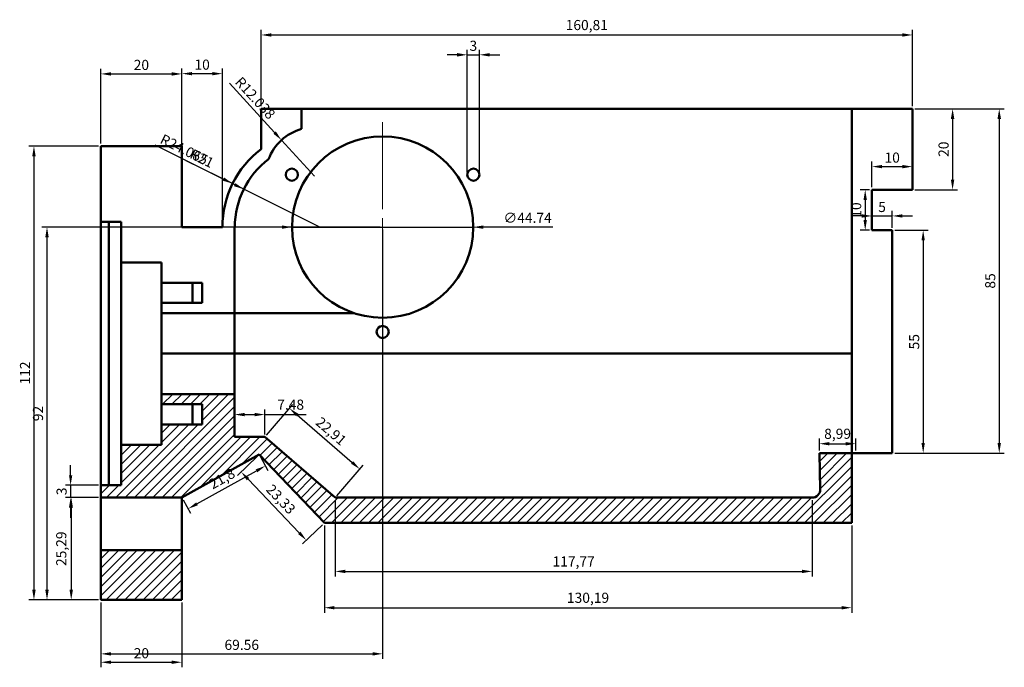
# Model space of a CAD drawing. Units: millimetres. Extents: x 1194 to 1920, y 1729 to 2086.
# Tile 1 of 5: x 1237 to 1480, y 1732 to 1891. Entities that reach past the tile are written whole.
import ezdxf

# ---------------------------------------------------------------- set-up
doc = ezdxf.new("R2010")
doc.units = ezdxf.units.MM
doc.linetypes.add('CENTER', pattern=[50.8, 31.75, -6.35, 6.35, -6.35])
for name, color, linetype, lineweight in [('M-CNTR', 1, 'CENTER', 18), ('M-DIMS', 2, 'Continuous', 25), ('M-HATC', 8, 'Continuous', 18), ('M-OUTL', 7, 'Continuous', 50)]:
    doc.layers.add(name, color=color, linetype=linetype, lineweight=lineweight)
doc.styles.get("Standard").update_dxf_attribs({"font": 'arial.ttf'})
doc.dimstyles.new('ISO-25', dxfattribs={"dimtxt": 2.5, "dimasz": 2.5, "dimexe": 1.25, "dimexo": 0.625, "dimtad": 1, "dimtxsty": 'Standard', "dimcen": 2.5, "dimadec": 0, "dimazin": 0, "dimtfac": 1, "dimtmove": 0, "dimatfit": 3, "dimfxl": 1, "dimarcsym": 0})

# ---------------------------------------------------------------- blocks, each defined once
blk = doc.blocks.new('*U10')
at = {"layer": 'M-CNTR', "color": 0, "transparency": 16777216}
for p, q in [((0, 4.47), (0, 25.87)), ((-25.87, 0), (-4.47, 0)), ((4.47, 0), (25.87, 0)), ((0, -25.87), (0, -4.47))]:
    blk.add_line(p, q, dxfattribs=at)
at = {"layer": 'M-CNTR', "color": 0, "linetype": 'Continuous', "transparency": 16777216}
for p, q in [((-2.24, 0), (2.24, 0)), ((0, -2.24), (0, 2.24))]:
    blk.add_line(p, q, dxfattribs=at)
blk = doc.blocks.new('*U11')
blk.add_circle((0, 0), 1.5)
blk = doc.blocks.new('*U12')
at = {"layer": 'M-OUTL', "color": 0, "linetype": 'ByBlock', "lineweight": -2, "transparency": 16777216}
for p, rotation in [((1304.02, 1853.17), 240), ((1348.83, 1853.17), 119.9999999999999)]:
    blk.add_blockref('*U11', p, dxfattribs=dict(at, rotation=rotation))
blk.add_blockref('*U11', (1326.43, 1814.36), dxfattribs=at)
blk = doc.blocks.new('*D81')
at = {"layer": 'Defpoints', "color": 0, "transparency": 16777216}
for p in [(1256.87, 1860.23), (1240.35, 1748.23), (1256.87, 1748.23)]:
    blk.add_point(p, dxfattribs=at)
at = {"layer": 'M-DIMS', "color": 0, "lineweight": -2, "transparency": 16777216}
for p, q in [((1256.25, 1860.23), (1239.1, 1860.23)), ((1240.35, 1857.73), (1240.35, 1750.73)), ((1256.25, 1748.23), (1239.1, 1748.23))]:
    blk.add_line(p, q, dxfattribs=at)
at = {"layer": 'M-DIMS', "color": 0, "transparency": 16777216}
for points in [[(1239.93, 1857.73), (1240.76, 1857.73), (1240.35, 1860.23)], [(1239.93, 1750.73), (1240.76, 1750.73), (1240.35, 1748.23)]]:
    blk.add_solid(points, dxfattribs=at)
at = {"layer": 'M-DIMS', "color": 0, "transparency": 16777216, "insert": (1238.47, 1804.23), "char_height": 2.5, "attachment_point": 5, "rotation": 90}
blk.add_mtext('112', dxfattribs=at)
blk = doc.blocks.new('*D82')
at = {"layer": 'Defpoints', "color": 0, "transparency": 16777216}
for p in [(1276.87, 1878.03), (1256.87, 1860.23), (1276.87, 1860.23)]:
    blk.add_point(p, dxfattribs=at)
at = {"layer": 'M-DIMS', "color": 0, "lineweight": -2, "transparency": 16777216}
for p, q in [((1256.87, 1860.86), (1256.87, 1879.28)), ((1276.87, 1860.86), (1276.87, 1879.28)), ((1259.37, 1878.03), (1274.37, 1878.03))]:
    blk.add_line(p, q, dxfattribs=at)
at = {"layer": 'M-DIMS', "color": 0, "transparency": 16777216}
for points in [[(1259.37, 1878.45), (1259.37, 1877.61), (1256.87, 1878.03)], [(1274.37, 1878.45), (1274.37, 1877.61), (1276.87, 1878.03)]]:
    blk.add_solid(points, dxfattribs=at)
at = {"layer": 'M-DIMS', "color": 0, "transparency": 16777216, "insert": (1266.87, 1879.93), "char_height": 2.5, "attachment_point": 5}
blk.add_mtext('20', dxfattribs=at)
blk = doc.blocks.new('*D83')
at = {"layer": 'Defpoints', "color": 0, "transparency": 16777216}
for p in [(1457.23, 1887.64), (1296.43, 1869.45), (1457.23, 1869.45)]:
    blk.add_point(p, dxfattribs=at)
at = {"layer": 'M-DIMS', "color": 0, "lineweight": -2, "transparency": 16777216}
for p, q in [((1296.43, 1870.07), (1296.43, 1888.89)), ((1457.23, 1870.07), (1457.23, 1888.89)), ((1298.93, 1887.64), (1454.73, 1887.64))]:
    blk.add_line(p, q, dxfattribs=at)
at = {"layer": 'M-DIMS', "color": 0, "transparency": 16777216}
for points in [[(1298.93, 1888.06), (1298.93, 1887.23), (1296.43, 1887.64)], [(1454.73, 1888.06), (1454.73, 1887.23), (1457.23, 1887.64)]]:
    blk.add_solid(points, dxfattribs=at)
at = {"layer": 'M-DIMS', "color": 0, "transparency": 16777216, "insert": (1376.83, 1889.77), "char_height": 2.5, "attachment_point": 5}
blk.add_mtext('160,81', dxfattribs=at)
blk = doc.blocks.new('*D84')
at = {"layer": 'Defpoints', "color": 0, "transparency": 16777216}
for p in [(1286.87, 1878.1), (1276.87, 1840.23), (1286.87, 1840.23)]:
    blk.add_point(p, dxfattribs=at)
at = {"layer": 'M-DIMS', "color": 0, "lineweight": -2, "transparency": 16777216}
for p, q in [((1276.87, 1840.86), (1276.87, 1879.35)), ((1286.87, 1840.86), (1286.87, 1879.35)), ((1279.37, 1878.1), (1284.37, 1878.1))]:
    blk.add_line(p, q, dxfattribs=at)
at = {"layer": 'M-DIMS', "color": 0, "transparency": 16777216}
for points in [[(1279.37, 1878.51), (1279.37, 1877.68), (1276.87, 1878.1)], [(1284.37, 1878.51), (1284.37, 1877.68), (1286.87, 1878.1)]]:
    blk.add_solid(points, dxfattribs=at)
at = {"layer": 'M-DIMS', "color": 0, "transparency": 16777216, "insert": (1281.87, 1880), "char_height": 2.5, "attachment_point": 5}
blk.add_mtext('10', dxfattribs=at)
blk = doc.blocks.new('*D85')
at = {"layer": 'Defpoints', "color": 0, "transparency": 16777216}
for p in [(1256.87, 1748.23), (1276.87, 1748.23), (1276.87, 1732.86)]:
    blk.add_point(p, dxfattribs=at)
at = {"layer": 'M-DIMS', "color": 0, "lineweight": -2, "transparency": 16777216}
for p, q in [((1256.87, 1747.61), (1256.87, 1731.61)), ((1276.87, 1747.61), (1276.87, 1731.61)), ((1259.37, 1732.86), (1274.37, 1732.86))]:
    blk.add_line(p, q, dxfattribs=at)
at = {"layer": 'M-DIMS', "color": 0, "transparency": 16777216}
for points in [[(1259.37, 1733.28), (1259.37, 1732.45), (1256.87, 1732.86)], [(1274.37, 1733.28), (1274.37, 1732.45), (1276.87, 1732.86)]]:
    blk.add_solid(points, dxfattribs=at)
at = {"layer": 'M-DIMS', "color": 0, "transparency": 16777216, "insert": (1266.87, 1734.77), "char_height": 2.5, "attachment_point": 5}
blk.add_mtext('20', dxfattribs=at)
blk = doc.blocks.new('*D86')
at = {"layer": 'Defpoints', "color": 0, "transparency": 16777216}
for p in [(1256.87, 1773.52), (1249.55, 1748.23), (1256.87, 1748.23)]:
    blk.add_point(p, dxfattribs=at)
at = {"layer": 'M-DIMS', "color": 0, "lineweight": -2, "transparency": 16777216}
for p, q in [((1256.25, 1773.52), (1248.3, 1773.52)), ((1249.55, 1771.02), (1249.55, 1750.73)), ((1256.25, 1748.23), (1248.3, 1748.23))]:
    blk.add_line(p, q, dxfattribs=at)
at = {"layer": 'M-DIMS', "color": 0, "transparency": 16777216}
for points in [[(1249.13, 1771.02), (1249.97, 1771.02), (1249.55, 1773.52)], [(1249.13, 1750.73), (1249.97, 1750.73), (1249.55, 1748.23)]]:
    blk.add_solid(points, dxfattribs=at)
at = {"layer": 'M-DIMS', "color": 0, "transparency": 16777216, "insert": (1247.42, 1760.87), "char_height": 2.5, "attachment_point": 5, "rotation": 90}
blk.add_mtext('25,29', dxfattribs=at)
blk = doc.blocks.new('*D87')
at = {"layer": 'Defpoints', "color": 0, "transparency": 16777216}
for p in [(1256.87, 1776.52), (1249.4, 1773.52), (1256.87, 1773.52)]:
    blk.add_point(p, dxfattribs=at)
at = {"layer": 'M-DIMS', "color": 0, "lineweight": -2, "transparency": 16777216}
for p, q in [((1249.4, 1779.02), (1249.4, 1781.52)), ((1256.25, 1776.52), (1248.15, 1776.52)), ((1249.4, 1776.52), (1249.4, 1773.52)), ((1256.25, 1773.52), (1248.15, 1773.52)), ((1249.4, 1771.02), (1249.4, 1768.52))]:
    blk.add_line(p, q, dxfattribs=at)
at = {"layer": 'M-DIMS', "color": 0, "transparency": 16777216}
for points in [[(1248.99, 1779.02), (1249.82, 1779.02), (1249.4, 1776.52)], [(1248.99, 1771.02), (1249.82, 1771.02), (1249.4, 1773.52)]]:
    blk.add_solid(points, dxfattribs=at)
at = {"layer": 'M-DIMS', "color": 0, "transparency": 16777216, "insert": (1247.5, 1775.02), "char_height": 2.5, "attachment_point": 5, "rotation": 90}
blk.add_mtext('3', dxfattribs=at)
blk = doc.blocks.new('*D88')
at = {"layer": 'Defpoints', "color": 0, "transparency": 16777216}
for p in [(1295.93, 1784.1), (1297.48, 1781.31), (1276.87, 1773.52)]:
    blk.add_point(p, dxfattribs=at)
at = {"layer": 'M-DIMS', "color": 0, "lineweight": -2, "transparency": 16777216}
for p, q in [((1296.24, 1783.55), (1298.09, 1780.21)), ((1280.6, 1771.94), (1295.3, 1780.09)), ((1277.17, 1772.97), (1279.02, 1769.64))]:
    blk.add_line(p, q, dxfattribs=at)
at = {"layer": 'M-DIMS', "color": 0, "transparency": 16777216}
for points in [[(1295.09, 1780.46), (1295.5, 1779.73), (1297.48, 1781.31)], [(1280.4, 1772.31), (1280.81, 1771.58), (1278.42, 1770.73)]]:
    blk.add_solid(points, dxfattribs=at)
at = {"layer": 'M-DIMS', "color": 0, "transparency": 16777216, "insert": (1286.92, 1777.88), "char_height": 2.5, "attachment_point": 5, "rotation": 29.0232}
blk.add_mtext('21,8', dxfattribs=at)
blk = doc.blocks.new('*D89')
at = {"layer": 'Defpoints', "color": 0, "transparency": 16777216}
for p in [(1295.93, 1784.1), (1312.04, 1767.22), (1307.59, 1762.97)]:
    blk.add_point(p, dxfattribs=at)
at = {"layer": 'M-DIMS', "color": 0, "lineweight": -2, "transparency": 16777216}
for p, q in [((1295.48, 1783.66), (1290.57, 1778.98)), ((1293.2, 1778.03), (1305.86, 1764.77)), ((1311.59, 1766.79), (1306.68, 1762.1))]:
    blk.add_line(p, q, dxfattribs=at)
at = {"layer": 'M-DIMS', "color": 0, "transparency": 16777216}
for points in [[(1293.51, 1778.32), (1292.9, 1777.75), (1291.48, 1779.84)], [(1306.16, 1765.06), (1305.56, 1764.49), (1307.59, 1762.97)]]:
    blk.add_solid(points, dxfattribs=at)
at = {"layer": 'M-DIMS', "color": 0, "transparency": 16777216, "insert": (1301.07, 1772.87), "char_height": 2.5, "attachment_point": 5, "rotation": 313.6718}
blk.add_mtext('23,33', dxfattribs=at)
blk = doc.blocks.new('*D90')
at = {"layer": 'Defpoints', "color": 0, "transparency": 16777216}
for p in [(1297.35, 1788.44), (1320.78, 1780.53), (1314.69, 1773.48)]:
    blk.add_point(p, dxfattribs=at)
at = {"layer": 'M-DIMS', "color": 0, "lineweight": -2, "transparency": 16777216}
for p, q in [((1297.76, 1788.91), (1304.26, 1796.45)), ((1305.33, 1793.87), (1318.89, 1782.17)), ((1315.1, 1773.95), (1321.6, 1781.48))]:
    blk.add_line(p, q, dxfattribs=at)
at = {"layer": 'M-DIMS', "color": 0, "transparency": 16777216}
for points in [[(1305.61, 1794.18), (1305.06, 1793.55), (1303.44, 1795.5)], [(1319.16, 1782.48), (1318.62, 1781.85), (1320.78, 1780.53)]]:
    blk.add_solid(points, dxfattribs=at)
at = {"layer": 'M-DIMS', "color": 0, "transparency": 16777216, "insert": (1313.5, 1789.63), "char_height": 2.5, "attachment_point": 5, "rotation": 319.2097}
blk.add_mtext('22,91', dxfattribs=at)
blk = doc.blocks.new('*D91')
at = {"layer": 'Defpoints', "color": 0, "transparency": 16777216}
for p in [(1297.35, 1793.97), (1289.87, 1788.44), (1297.35, 1788.44)]:
    blk.add_point(p, dxfattribs=at)
at = {"layer": 'M-DIMS', "color": 0, "lineweight": -2, "transparency": 16777216}
for p, q in [((1289.87, 1789.07), (1289.87, 1795.22)), ((1292.37, 1793.97), (1294.85, 1793.97)), ((1297.35, 1789.07), (1297.35, 1795.22)), ((1297.35, 1793.97), (1307.58, 1793.97))]:
    blk.add_line(p, q, dxfattribs=at)
at = {"layer": 'M-DIMS', "color": 0, "transparency": 16777216}
for points in [[(1292.37, 1794.39), (1292.37, 1793.56), (1289.87, 1793.97)], [(1294.85, 1794.39), (1294.85, 1793.56), (1297.35, 1793.97)]]:
    blk.add_solid(points, dxfattribs=at)
at = {"layer": 'M-DIMS', "color": 0, "transparency": 16777216, "insert": (1303.72, 1796.1), "char_height": 2.5, "attachment_point": 5}
blk.add_mtext('7,48', dxfattribs=at)
blk = doc.blocks.new('*D92')
at = {"layer": 'Defpoints', "color": 0, "transparency": 16777216}
for p in [(1312.04, 1767.22), (1442.23, 1767.22), (1442.23, 1746.31)]:
    blk.add_point(p, dxfattribs=at)
at = {"layer": 'M-DIMS', "color": 0, "lineweight": -2, "transparency": 16777216}
for p, q in [((1312.04, 1766.6), (1312.04, 1745.06)), ((1442.23, 1766.6), (1442.23, 1745.06)), ((1314.54, 1746.31), (1439.73, 1746.31))]:
    blk.add_line(p, q, dxfattribs=at)
at = {"layer": 'M-DIMS', "color": 0, "transparency": 16777216}
for points in [[(1314.54, 1746.73), (1314.54, 1745.89), (1312.04, 1746.31)], [(1439.73, 1746.73), (1439.73, 1745.89), (1442.23, 1746.31)]]:
    blk.add_solid(points, dxfattribs=at)
at = {"layer": 'M-DIMS', "color": 0, "transparency": 16777216, "insert": (1377.14, 1748.44), "char_height": 2.5, "attachment_point": 5}
blk.add_mtext('130,19', dxfattribs=at)
blk = doc.blocks.new('*D93')
at = {"layer": 'Defpoints', "color": 0, "transparency": 16777216}
for p in [(1314.69, 1773.48), (1432.47, 1773.48), (1432.47, 1755.27)]:
    blk.add_point(p, dxfattribs=at)
at = {"layer": 'M-DIMS', "color": 0, "lineweight": -2, "transparency": 16777216}
for p, q in [((1314.69, 1772.85), (1314.69, 1754.02)), ((1432.47, 1772.85), (1432.47, 1754.02)), ((1317.19, 1755.27), (1429.97, 1755.27))]:
    blk.add_line(p, q, dxfattribs=at)
at = {"layer": 'M-DIMS', "color": 0, "transparency": 16777216}
for points in [[(1317.19, 1755.69), (1317.19, 1754.86), (1314.69, 1755.27)], [(1429.97, 1755.69), (1429.97, 1754.86), (1432.47, 1755.27)]]:
    blk.add_solid(points, dxfattribs=at)
at = {"layer": 'M-DIMS', "color": 0, "transparency": 16777216, "insert": (1373.58, 1757.4), "char_height": 2.5, "attachment_point": 5}
blk.add_mtext('117,77', dxfattribs=at)
blk = doc.blocks.new('*D94')
at = {"layer": 'Defpoints', "color": 0, "transparency": 16777216}
for p in [(1443.24, 1786.78), (1434.25, 1784.45), (1443.24, 1784.45)]:
    blk.add_point(p, dxfattribs=at)
at = {"layer": 'M-DIMS', "color": 0, "lineweight": -2, "transparency": 16777216}
for p, q in [((1434.25, 1785.07), (1434.25, 1788.03)), ((1436.75, 1786.78), (1440.74, 1786.78)), ((1443.24, 1785.07), (1443.24, 1788.03))]:
    blk.add_line(p, q, dxfattribs=at)
at = {"layer": 'M-DIMS', "color": 0, "transparency": 16777216}
for points in [[(1436.75, 1787.2), (1436.75, 1786.36), (1434.25, 1786.78)], [(1440.74, 1787.2), (1440.74, 1786.36), (1443.24, 1786.78)]]:
    blk.add_solid(points, dxfattribs=at)
at = {"layer": 'M-DIMS', "color": 0, "transparency": 16777216, "insert": (1438.75, 1788.91), "char_height": 2.5, "attachment_point": 5}
blk.add_mtext('8,99', dxfattribs=at)
blk = doc.blocks.new('*D95')
at = {"layer": 'Defpoints', "color": 0, "transparency": 16777216}
for p in [(1457.23, 1869.45), (1452.23, 1784.45), (1478.66, 1784.45)]:
    blk.add_point(p, dxfattribs=at)
at = {"layer": 'M-DIMS', "color": 0, "lineweight": -2, "transparency": 16777216}
for p, q in [((1457.86, 1869.45), (1479.91, 1869.45)), ((1478.66, 1866.95), (1478.66, 1786.95)), ((1452.86, 1784.45), (1479.91, 1784.45))]:
    blk.add_line(p, q, dxfattribs=at)
at = {"layer": 'M-DIMS', "color": 0, "transparency": 16777216}
for points in [[(1478.24, 1866.95), (1479.08, 1866.95), (1478.66, 1869.45)], [(1478.24, 1786.95), (1479.08, 1786.95), (1478.66, 1784.45)]]:
    blk.add_solid(points, dxfattribs=at)
at = {"layer": 'M-DIMS', "color": 0, "transparency": 16777216, "insert": (1476.76, 1826.95), "char_height": 2.5, "attachment_point": 5, "rotation": 90}
blk.add_mtext('85', dxfattribs=at)
blk = doc.blocks.new('*D96')
at = {"layer": 'Defpoints', "color": 0, "transparency": 16777216}
for p in [(1457.23, 1869.45), (1457.23, 1849.45), (1467.14, 1849.45)]:
    blk.add_point(p, dxfattribs=at)
at = {"layer": 'M-DIMS', "color": 0, "lineweight": -2, "transparency": 16777216}
for p, q in [((1457.86, 1869.45), (1468.39, 1869.45)), ((1467.14, 1866.95), (1467.14, 1851.95)), ((1457.86, 1849.45), (1468.39, 1849.45))]:
    blk.add_line(p, q, dxfattribs=at)
at = {"layer": 'M-DIMS', "color": 0, "transparency": 16777216}
for points in [[(1466.72, 1866.95), (1467.56, 1866.95), (1467.14, 1869.45)], [(1466.72, 1851.95), (1467.56, 1851.95), (1467.14, 1849.45)]]:
    blk.add_solid(points, dxfattribs=at)
at = {"layer": 'M-DIMS', "color": 0, "transparency": 16777216, "insert": (1465.24, 1859.45), "char_height": 2.5, "attachment_point": 5, "rotation": 90}
blk.add_mtext('20', dxfattribs=at)
blk = doc.blocks.new('*D97')
at = {"layer": 'Defpoints', "color": 0, "transparency": 16777216}
for p in [(1457.23, 1855.16), (1447.23, 1849.45), (1457.23, 1849.45)]:
    blk.add_point(p, dxfattribs=at)
at = {"layer": 'M-DIMS', "color": 0, "lineweight": -2, "transparency": 16777216}
for p, q in [((1447.23, 1850.07), (1447.23, 1856.41)), ((1449.73, 1855.16), (1454.73, 1855.16)), ((1457.23, 1850.07), (1457.23, 1856.41))]:
    blk.add_line(p, q, dxfattribs=at)
at = {"layer": 'M-DIMS', "color": 0, "transparency": 16777216}
for points in [[(1449.73, 1855.58), (1449.73, 1854.74), (1447.23, 1855.16)], [(1454.73, 1855.58), (1454.73, 1854.74), (1457.23, 1855.16)]]:
    blk.add_solid(points, dxfattribs=at)
at = {"layer": 'M-DIMS', "color": 0, "transparency": 16777216, "insert": (1452.23, 1857.06), "char_height": 2.5, "attachment_point": 5}
blk.add_mtext('10', dxfattribs=at)
blk = doc.blocks.new('*D98')
at = {"layer": 'Defpoints', "color": 0, "transparency": 16777216}
for p in [(1447.23, 1849.45), (1445.57, 1839.45), (1447.23, 1839.45)]:
    blk.add_point(p, dxfattribs=at)
at = {"layer": 'M-DIMS', "color": 0, "lineweight": -2, "transparency": 16777216}
for p, q in [((1446.61, 1849.45), (1444.32, 1849.45)), ((1445.57, 1846.95), (1445.57, 1841.95)), ((1446.61, 1839.45), (1444.32, 1839.45))]:
    blk.add_line(p, q, dxfattribs=at)
at = {"layer": 'M-DIMS', "color": 0, "transparency": 16777216}
for points in [[(1445.15, 1846.95), (1445.98, 1846.95), (1445.57, 1849.45)], [(1445.15, 1841.95), (1445.98, 1841.95), (1445.57, 1839.45)]]:
    blk.add_solid(points, dxfattribs=at)
at = {"layer": 'M-DIMS', "color": 0, "transparency": 16777216, "insert": (1443.66, 1844.45), "char_height": 2.5, "attachment_point": 5, "rotation": 90}
blk.add_mtext('10', dxfattribs=at)
blk = doc.blocks.new('*D99')
at = {"layer": 'Defpoints', "color": 0, "transparency": 16777216}
for p in [(1452.23, 1842.99), (1447.23, 1839.45), (1452.23, 1839.45)]:
    blk.add_point(p, dxfattribs=at)
at = {"layer": 'M-DIMS', "color": 0, "lineweight": -2, "transparency": 16777216}
for p, q in [((1444.73, 1842.99), (1442.23, 1842.99)), ((1447.23, 1840.07), (1447.23, 1844.24)), ((1447.23, 1842.99), (1452.23, 1842.99)), ((1452.23, 1840.07), (1452.23, 1844.24)), ((1454.73, 1842.99), (1457.23, 1842.99))]:
    blk.add_line(p, q, dxfattribs=at)
at = {"layer": 'M-DIMS', "color": 0, "transparency": 16777216}
for points in [[(1444.73, 1843.4), (1444.73, 1842.57), (1447.23, 1842.99)], [(1454.73, 1843.4), (1454.73, 1842.57), (1452.23, 1842.99)]]:
    blk.add_solid(points, dxfattribs=at)
at = {"layer": 'M-DIMS', "color": 0, "transparency": 16777216, "insert": (1449.73, 1844.88), "char_height": 2.5, "attachment_point": 5}
blk.add_mtext('5', dxfattribs=at)
blk = doc.blocks.new('*D100')
at = {"layer": 'Defpoints', "color": 0, "transparency": 16777216}
for p in [(1452.23, 1839.45), (1452.23, 1784.45), (1459.88, 1784.45)]:
    blk.add_point(p, dxfattribs=at)
at = {"layer": 'M-DIMS', "color": 0, "lineweight": -2, "transparency": 16777216}
for p, q in [((1452.86, 1839.45), (1461.13, 1839.45)), ((1459.88, 1836.95), (1459.88, 1786.95)), ((1452.86, 1784.45), (1461.13, 1784.45))]:
    blk.add_line(p, q, dxfattribs=at)
at = {"layer": 'M-DIMS', "color": 0, "transparency": 16777216}
for points in [[(1459.46, 1836.95), (1460.29, 1836.95), (1459.88, 1839.45)], [(1459.46, 1786.95), (1460.29, 1786.95), (1459.88, 1784.45)]]:
    blk.add_solid(points, dxfattribs=at)
at = {"layer": 'M-DIMS', "color": 0, "transparency": 16777216, "insert": (1457.98, 1811.95), "char_height": 2.5, "attachment_point": 5, "rotation": 90}
blk.add_mtext('55', dxfattribs=at)
blk = doc.blocks.new('*D138')
at = {"layer": 'Defpoints', "color": 0, "transparency": 16777216}
for p in [(1350.33, 1882.75), (1347.33, 1853.17), (1350.33, 1853.17)]:
    blk.add_point(p, dxfattribs=at)
at = {"layer": 'M-DIMS', "color": 0, "lineweight": -2, "transparency": 16777216}
for p, q in [((1347.33, 1853.79), (1347.33, 1884)), ((1350.33, 1853.79), (1350.33, 1884)), ((1344.83, 1882.75), (1342.33, 1882.75)), ((1347.33, 1882.75), (1350.33, 1882.75)), ((1352.83, 1882.75), (1355.33, 1882.75))]:
    blk.add_line(p, q, dxfattribs=at)
at = {"layer": 'M-DIMS', "color": 0, "transparency": 16777216}
for points in [[(1344.83, 1883.17), (1344.83, 1882.33), (1347.33, 1882.75)], [(1352.83, 1883.17), (1352.83, 1882.33), (1350.33, 1882.75)]]:
    blk.add_solid(points, dxfattribs=at)
at = {"layer": 'M-DIMS', "color": 0, "transparency": 16777216, "insert": (1348.83, 1884.65), "char_height": 2.5, "attachment_point": 5}
blk.add_mtext('3', dxfattribs=at)
blk = doc.blocks.new('*D142')
at = {"layer": 'Defpoints', "color": 0, "transparency": 16777216}
for p in [(1326.43, 1840.23), (1256.87, 1748.23), (1326.43, 1734.93)]:
    blk.add_point(p, dxfattribs=at)
at = {"layer": 'M-DIMS', "color": 0, "lineweight": -2, "transparency": 16777216}
for p, q in [((1326.43, 1839.61), (1326.43, 1733.68)), ((1256.87, 1747.61), (1256.87, 1733.68)), ((1259.37, 1734.93), (1323.93, 1734.93))]:
    blk.add_line(p, q, dxfattribs=at)
at = {"layer": 'M-DIMS', "color": 0, "transparency": 16777216}
for points in [[(1259.37, 1735.35), (1259.37, 1734.51), (1256.87, 1734.93)], [(1323.93, 1735.35), (1323.93, 1734.51), (1326.43, 1734.93)]]:
    blk.add_solid(points, dxfattribs=at)
at = {"layer": 'M-DIMS', "color": 0, "transparency": 16777216, "insert": (1291.65, 1736.83), "char_height": 2.5, "attachment_point": 5}
blk.add_mtext('69.56', dxfattribs=at)
blk = doc.blocks.new('*D143')
at = {"layer": 'Defpoints', "color": 0, "transparency": 16777216}
for p in [(1243.57, 1840.23), (1326.43, 1840.23), (1256.87, 1748.23)]:
    blk.add_point(p, dxfattribs=at)
at = {"layer": 'M-DIMS', "color": 0, "lineweight": -2, "transparency": 16777216}
for p, q in [((1325.8, 1840.23), (1242.32, 1840.23)), ((1243.57, 1750.73), (1243.57, 1837.73)), ((1256.25, 1748.23), (1242.32, 1748.23))]:
    blk.add_line(p, q, dxfattribs=at)
at = {"layer": 'M-DIMS', "color": 0, "transparency": 16777216}
for points in [[(1243.15, 1837.73), (1243.99, 1837.73), (1243.57, 1840.23)], [(1243.15, 1750.73), (1243.99, 1750.73), (1243.57, 1748.23)]]:
    blk.add_solid(points, dxfattribs=at)
at = {"layer": 'M-DIMS', "color": 0, "transparency": 16777216, "insert": (1241.67, 1794.23), "char_height": 2.5, "attachment_point": 5, "rotation": 90}
blk.add_mtext('92', dxfattribs=at)
blk = doc.blocks.new('*D150')
at = {"layer": 'Defpoints', "color": 0, "transparency": 16777216}
for p in [(1304.05, 1840.23), (1348.8, 1840.23)]:
    blk.add_point(p, dxfattribs=at)
at = {"layer": 'M-DIMS', "color": 0, "lineweight": -2, "transparency": 16777216}
for p, q in [((1301.55, 1840.23), (1299.05, 1840.23)), ((1304.05, 1840.23), (1348.8, 1840.23)), ((1368.42, 1840.23), (1351.3, 1840.23))]:
    blk.add_line(p, q, dxfattribs=at)
at = {"layer": 'M-DIMS', "color": 0, "transparency": 16777216}
for points in [[(1301.55, 1840.65), (1301.55, 1839.81), (1304.05, 1840.23)], [(1351.3, 1840.65), (1351.3, 1839.81), (1348.8, 1840.23)]]:
    blk.add_solid(points, dxfattribs=at)
at = {"layer": 'M-DIMS', "color": 0, "transparency": 16777216, "insert": (1362.22, 1842.2), "char_height": 2.5, "attachment_point": 5, "rotation": 359.9989}
blk.add_mtext('∅44.74', dxfattribs=at)
blk = doc.blocks.new('*D151')
at = {"layer": 'Defpoints', "color": 0, "transparency": 16777216}
for p in [(1289.39, 1850.96), (1310.94, 1840.25)]:
    blk.add_point(p, dxfattribs=at)
at = {"layer": 'M-DIMS', "color": 0, "lineweight": -2, "transparency": 16777216}
for p, q in [((1270.17, 1860.52), (1287.15, 1852.08)), ((1310.94, 1840.25), (1289.39, 1850.96))]:
    blk.add_line(p, q, dxfattribs=at)
at = {"layer": 'M-DIMS', "color": 0, "transparency": 16777216}
blk.add_solid([(1287.33, 1852.45), (1286.96, 1851.7), (1289.39, 1850.96)], dxfattribs=at)
at = {"layer": 'M-DIMS', "color": 0, "transparency": 16777216, "insert": (1277.3, 1859.1), "char_height": 2.5, "attachment_point": 5, "rotation": 333.5623}
blk.add_mtext('R24.065', dxfattribs=at)
blk = doc.blocks.new('*D152')
at = {"layer": 'Defpoints', "color": 0, "transparency": 16777216}
for p in [(1292.13, 1849.6), (1310.94, 1840.25)]:
    blk.add_point(p, dxfattribs=at)
at = {"layer": 'M-DIMS', "color": 0, "lineweight": -2, "transparency": 16777216}
for p, q in [((1277.83, 1856.71), (1289.9, 1850.71)), ((1310.94, 1840.25), (1292.13, 1849.6))]:
    blk.add_line(p, q, dxfattribs=at)
at = {"layer": 'M-DIMS', "color": 0, "transparency": 16777216}
blk.add_solid([(1290.08, 1851.08), (1289.71, 1850.34), (1292.13, 1849.6)], dxfattribs=at)
at = {"layer": 'M-DIMS', "color": 0, "transparency": 16777216, "insert": (1281.69, 1856.89), "char_height": 2.5, "attachment_point": 5, "rotation": 333.5627}
blk.add_mtext('R21', dxfattribs=at)
blk = doc.blocks.new('*D153')
at = {"layer": 'Defpoints', "color": 0, "transparency": 16777216}
for p in [(1301.45, 1861.71), (1309.57, 1852.83)]:
    blk.add_point(p, dxfattribs=at)
at = {"layer": 'M-DIMS', "color": 0, "lineweight": -2, "transparency": 16777216}
for p, q in [((1288.61, 1875.76), (1299.76, 1863.56)), ((1309.57, 1852.83), (1301.45, 1861.71))]:
    blk.add_line(p, q, dxfattribs=at)
at = {"layer": 'M-DIMS', "color": 0, "transparency": 16777216}
blk.add_solid([(1300.07, 1863.84), (1299.45, 1863.28), (1301.45, 1861.71)], dxfattribs=at)
at = {"layer": 'M-DIMS', "color": 0, "transparency": 16777216, "insert": (1294.75, 1871.87), "char_height": 2.5, "attachment_point": 5, "rotation": 312.417}
blk.add_mtext('R12.038', dxfattribs=at)

msp = doc.modelspace()

# ---------------------------------------------------------------- hatches: boundary and pattern name
at = {"layer": 'M-HATC'}
h = msp.add_hatch(dxfattribs=at)
h.set_pattern_fill('ANSI31', color=256, scale=0.51)
h.paths.add_polyline_path([(1297.3519, 1788.4411), (1289.8705, 1788.4411), (1289.8705, 1799.019), (1271.8705, 1799.019), (1271.8705, 1796.519), (1281.8705, 1796.519), (1281.8705, 1791.519), (1271.8705, 1791.519), (1271.8705, 1786.519), (1261.8705, 1786.519), (1261.8705, 1776.519), (1256.8705, 1776.519), (1256.8705, 1773.519), (1276.8705, 1773.519), (1295.9338, 1784.096), (1312.0447, 1767.2203), (1442.2312, 1767.2203), (1442.2312, 1784.4485), (1434.2534, 1784.4485), (1434.4671, 1775.5243, -0.42124399), (1432.4677, 1773.4765), (1314.6945, 1773.4765)])
h.paths.add_polyline_path([(1276.8705, 1760.4931), (1256.8705, 1760.4931), (1256.8705, 1748.2304), (1276.8705, 1748.2304)])

# ---------------------------------------------------------------- linework, layer by layer
at = {"layer": 'M-OUTL'}
for p, q in [((1296.426, 1859.4485), (1296.426, 1869.4485)), ((1296.426, 1869.4485), (1442.2312, 1869.4485)), ((1296.426, 1869.4485), (1306.426, 1869.4485)), ((1296.426, 1869.4485), (1326.426, 1869.4485)), ((1306.426, 1869.4485), (1306.426, 1864.4485)), ((1442.2312, 1767.2203), (1442.2312, 1869.4485)), ((1442.2312, 1869.4485), (1457.2312, 1869.4485)), ((1457.2312, 1869.4485), (1457.2312, 1849.4485)), ((1256.8705, 1860.2304), (1256.8705, 1748.2304)), ((1276.8705, 1860.2304), (1256.8705, 1860.2304)), ((1276.8705, 1860.2304), (1276.8705, 1840.2304)), ((1457.2312, 1849.4485), (1447.2312, 1849.4485)), ((1447.2312, 1849.4485), (1447.2312, 1839.4485)), ((1261.8705, 1841.519), (1256.8705, 1841.519)), ((1258.8192, 1841.519), (1258.8192, 1776.519)), ((1261.8705, 1776.519), (1261.8705, 1841.519)), ((1261.8705, 1841.519), (1261.8705, 1831.519)), ((1276.8705, 1840.2304), (1286.8705, 1840.2304)), ((1289.8705, 1819.019), (1289.8705, 1840.1719)), ((1447.2312, 1839.4485), (1452.2312, 1839.4485)), ((1452.2312, 1839.4485), (1452.2312, 1784.4485)), ((1261.8705, 1831.519), (1271.8705, 1831.519)), ((1271.8705, 1831.519), (1271.8705, 1786.519)), ((1271.8705, 1831.519), (1271.8705, 1826.519)), ((1271.8705, 1826.519), (1281.8705, 1826.519)), ((1279.4543, 1826.519), (1279.4543, 1821.519)), ((1281.8705, 1826.519), (1281.8705, 1821.519)), ((1281.8705, 1821.519), (1271.8705, 1821.519)), ((1271.8705, 1809.019), (1271.8705, 1819.019)), ((1271.8705, 1819.019), (1289.8705, 1819.019)), ((1289.8705, 1819.019), (1289.8705, 1799.019)), ((1289.8705, 1819.019), (1304.8705, 1819.019)), ((1304.8705, 1819.019), (1319.3157, 1819.019)), ((1271.8705, 1809.019), (1442.2312, 1809.019)), ((1289.8705, 1799.019), (1271.8705, 1799.019)), ((1289.8705, 1799.019), (1289.8705, 1788.4411)), ((1281.8705, 1796.519), (1271.8705, 1796.519)), ((1279.4543, 1796.519), (1279.4543, 1791.519)), ((1281.8705, 1791.519), (1281.8705, 1796.519)), ((1271.8705, 1786.519), (1271.8705, 1791.519)), ((1271.8705, 1791.519), (1281.8705, 1791.519)), ((1289.8705, 1788.4411), (1297.3519, 1788.4411)), ((1297.3519, 1788.4411), (1314.6945, 1773.4765)), ((1261.8705, 1776.519), (1261.8705, 1786.519)), ((1261.8705, 1786.519), (1271.8705, 1786.519)), ((1452.2312, 1784.4485), (1434.2534, 1784.4485)), ((1434.4671, 1775.5243), (1434.2534, 1784.4485)), ((1276.8705, 1773.519), (1295.9338, 1784.096)), ((1295.9338, 1784.096), (1312.0447, 1767.2203)), ((1256.8705, 1773.519), (1256.8705, 1776.519)), ((1256.8705, 1776.519), (1261.8705, 1776.519)), ((1276.8705, 1773.519), (1256.8705, 1773.519)), ((1276.8705, 1748.2304), (1276.8705, 1773.519)), ((1314.6945, 1773.4765), (1432.4677, 1773.4765)), ((1312.0447, 1767.2203), (1442.2312, 1767.2203)), ((1256.8705, 1760.4931), (1276.8705, 1760.4931)), ((1256.8705, 1748.2304), (1276.8705, 1748.2304))]:
    msp.add_line(p, q, dxfattribs=at)
msp.add_circle((1326.426, 1840.2304), 22.3715, dxfattribs=at)
for centre, radius, start, end in [((1309.5667, 1852.8271), 12.0383, 105.122964, 159.710621), ((1310.9359, 1840.2494), 24.0654, 127.080482, 180.045103), ((1310.9359, 1840.2494), 20.9982, 127.080482, 180.045103), ((1432.4677, 1775.4765), 2, 270, 1.371866)]:
    msp.add_arc(centre, radius, start, end, dxfattribs=at)

# ---------------------------------------------------------------- block references
at = {"layer": 'M-CNTR'}
msp.add_blockref('*U10', (1326.426, 1840.2304), dxfattribs=at)
at = {"layer": 'M-OUTL'}
msp.add_blockref('*U12', (0, 0), dxfattribs=at)

# ---------------------------------------------------------------- dimensions: what is measured, and where the dimension line sits
at = {"layer": 'M-DIMS'}
for p1, p2, distance, picture, middle in [((1296.426, 1869.4485), (1457.2312, 1869.4485), 18.1954, '*D83', (1376.8286, 1889.7713)), ((1256.8705, 1860.2304), (1276.8705, 1860.2304), 17.7993, '*D82', (1266.8705, 1879.9312)), ((1276.8705, 1840.2304), (1286.8705, 1840.2304), 37.8659, '*D84', (1281.8705, 1879.9977)), ((1256.8705, 1860.2304), (1256.8705, 1748.2304), -16.5228, '*D81', (1238.4676, 1804.2304)), ((1297.3519, 1788.4411), (1314.6945, 1773.4765), 9.3223, '*D90', (1313.5032, 1789.6274)), ((1276.8705, 1773.519), (1295.9338, 1784.096), -3.1905, '*D88', (1286.918, 1777.8779)), ((1295.9338, 1784.096), (1312.0447, 1767.2203), -6.161, '*D89', (1301.0717, 1772.8728))]:
    dim = msp.add_aligned_dim(p1=p1, p2=p2, distance=distance, dimstyle='ISO-25', override={"dimclrd": 0, "dimclre": 0, "dimclrt": 0}, dxfattribs=at)
    dim.commit()
    dim.dimension.update_dxf_attribs({"geometry": picture, "text_midpoint": middle})
for base, p1, p2, override, picture, middle in [((1350.3314, 1882.7485), (1347.3314, 1853.1661), (1350.3314, 1853.1661), {"dimdec": 0, "dimlfac": 1, "dimrnd": 0, "dimzin": 0, "dimdsep": 46, "dimlunit": 2}, '*D138', (1348.8314, 1884.6508)), ((1457.2312, 1855.1599), (1447.2312, 1849.4485), (1457.2312, 1849.4485), {"dimclrd": 0, "dimclre": 0, "dimclrt": 0}, '*D97', (1452.2312, 1857.0614)), ((1452.2312, 1842.9865), (1447.2312, 1839.4485), (1452.2312, 1839.4485), {"dimclrd": 0, "dimclre": 0, "dimclrt": 0}, '*D99', (1449.7312, 1844.8828)), ((1326.426, 1734.9304), (1256.8705, 1748.2304), (1326.426, 1840.2304), {"dimdec": 2, "dimlfac": 1, "dimrnd": 0, "dimzin": 0, "dimdsep": 46, "dimlunit": 2}, '*D142', (1291.6483, 1736.8319)), ((1297.3519, 1793.9747), (1289.8705, 1788.4411), (1297.3519, 1788.4411), {"dimclrd": 0, "dimclre": 0, "dimclrt": 0}, '*D91', (1303.7162, 1796.1021)), ((1443.2423, 1786.7797), (1434.2534, 1784.4485), (1443.2423, 1784.4485), {"dimclrd": 0, "dimclre": 0, "dimclrt": 0}, '*D94', (1438.7479, 1788.9071)), ((1432.4677, 1755.2729), (1314.6945, 1773.4765), (1432.4677, 1773.4765), {"dimclrd": 0, "dimclre": 0, "dimclrt": 0}, '*D93', (1373.5811, 1757.4003)), ((1442.2312, 1746.3089), (1312.0447, 1767.2203), (1442.2312, 1767.2203), {"dimclrd": 0, "dimclre": 0, "dimclrt": 0}, '*D92', (1377.138, 1748.4362)), ((1276.8705, 1732.8636), (1256.8705, 1748.2304), (1276.8705, 1748.2304), {"dimclrd": 0, "dimclre": 0, "dimclrt": 0}, '*D85', (1266.8705, 1734.765))]:
    dim = msp.add_linear_dim(base=base, p1=p1, p2=p2, dimstyle='ISO-25', override=override, dxfattribs=at)
    dim.commit()
    dim.dimension.update_dxf_attribs({"geometry": picture, "text_midpoint": middle})
dim = msp.add_radius_dim(center=(1309.5667, 1852.8271), mpoint=(1301.4466, 1861.7144), dimstyle='ISO-25', override={"dimdec": 3, "dimlfac": 1, "dimrnd": 0, "dimzin": 0, "dimdsep": 46, "dimlunit": 2}, dxfattribs=at)
dim.commit()
dim.dimension.update_dxf_attribs({"geometry": '*D153', "text_midpoint": (1294.7479, 1871.8663)})
for base, p1, p2, override, picture, middle in [((1478.659, 1784.4485), (1457.2312, 1869.4485), (1452.2312, 1784.4485), {"dimclrd": 0, "dimclre": 0, "dimclrt": 0}, '*D95', (1476.7576, 1826.9485)), ((1467.1407, 1849.4485), (1457.2312, 1869.4485), (1457.2312, 1849.4485), {"dimclrd": 0, "dimclre": 0, "dimclrt": 0}, '*D96', (1465.2392, 1859.4485)), ((1445.566, 1839.4485), (1447.2312, 1849.4485), (1447.2312, 1839.4485), {"dimclrd": 0, "dimclre": 0, "dimclrt": 0}, '*D98', (1443.6646, 1844.4485)), ((1243.5705, 1840.2304), (1256.8705, 1748.2304), (1326.426, 1840.2304), {"dimdec": 0, "dimlfac": 1, "dimrnd": 0, "dimzin": 0, "dimdsep": 46, "dimlunit": 2}, '*D143', (1241.6691, 1794.2304)), ((1459.8777, 1784.4485), (1452.2312, 1839.4485), (1452.2312, 1784.4485), {"dimclrd": 0, "dimclre": 0, "dimclrt": 0}, '*D100', (1457.9814, 1811.9485)), ((1249.4046, 1773.519), (1256.8705, 1776.519), (1256.8705, 1773.519), {"dimclrd": 0, "dimclre": 0, "dimclrt": 0}, '*D87', (1247.5023, 1775.019)), ((1249.549, 1748.2304), (1256.8705, 1773.519), (1256.8705, 1748.2304), {"dimclrd": 0, "dimclre": 0, "dimclrt": 0}, '*D86', (1247.4217, 1760.8747))]:
    dim = msp.add_linear_dim(base=base, p1=p1, p2=p2, angle=90, dimstyle='ISO-25', override=override, dxfattribs=at)
    dim.commit()
    dim.dimension.update_dxf_attribs({"geometry": picture, "text_midpoint": middle})
for mpoint, override, picture, middle in [((1289.3873, 1850.9639), {"dimdec": 3, "dimlfac": 1, "dimrnd": 0, "dimzin": 0, "dimdsep": 46, "dimlunit": 2}, '*D151', (1276.4581, 1857.3925)), ((1292.1337, 1849.5982), {"dimdec": 0, "dimlfac": 1, "dimrnd": 0, "dimzin": 0, "dimdsep": 46, "dimlunit": 2}, '*D152', (1280.8523, 1855.2074))]:
    dim = msp.add_radius_dim(center=(1310.9359, 1840.2494), mpoint=mpoint, dimstyle='ISO-25', override=override, dxfattribs=at)
    dim.commit()
    dim.dimension.update_dxf_attribs({"geometry": picture, "text_midpoint": middle, "dimtype": 164})
dim = msp.add_diameter_dim_2p(p1=(1304.0546, 1840.2308), p2=(1348.7975, 1840.23), dimstyle='ISO-25', override={"dimdec": 2, "dimlfac": 1, "dimrnd": 0, "dimzin": 0, "dimdsep": 46, "dimlunit": 2}, dxfattribs=at)
dim.commit()
dim.dimension.update_dxf_attribs({"geometry": '*D150', "text_midpoint": (1362.2203, 1840.2297), "dimtype": 163})

doc.saveas('drawing.dxf')
